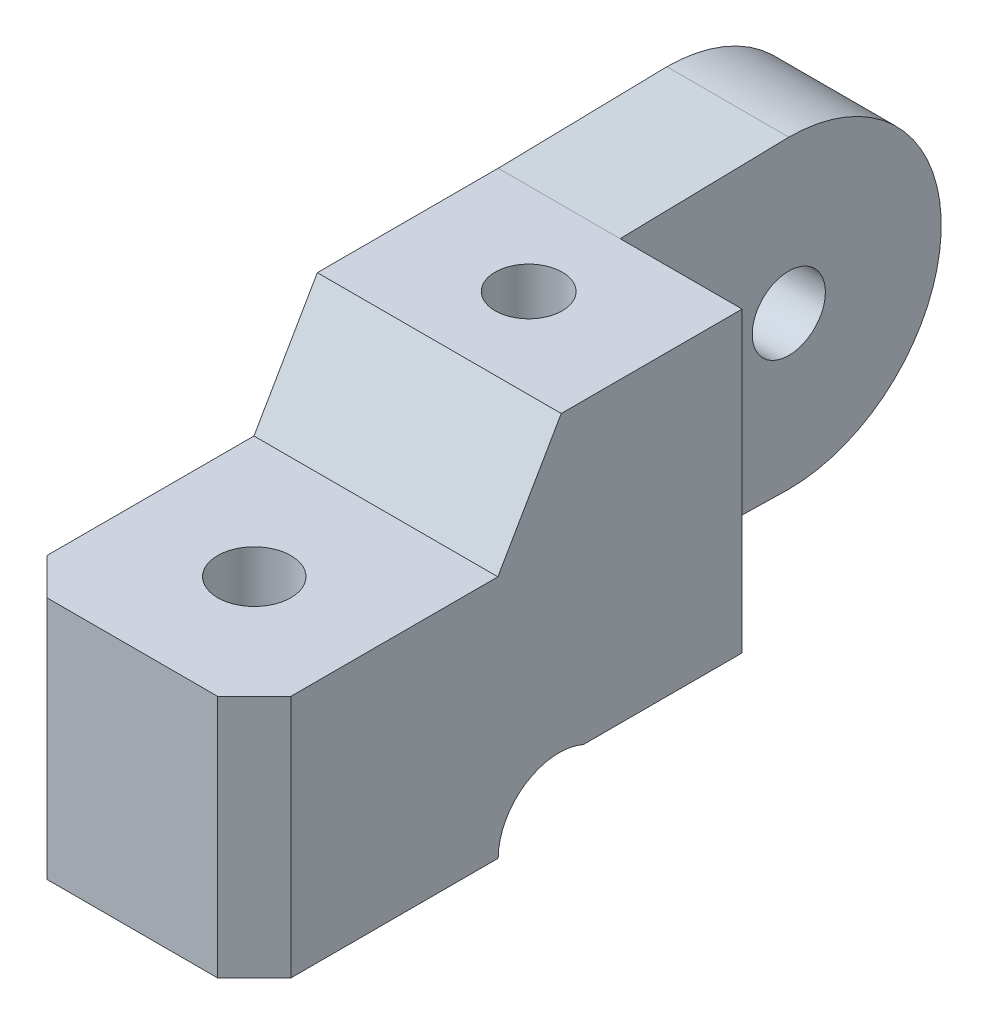
ISO-10303-21;
HEADER;
FILE_DESCRIPTION(('STEP AP214'),'2;1');
FILE_NAME('part.step','',(''),(''),'','','');
FILE_SCHEMA(('AUTOMOTIVE_DESIGN { 1 0 10303 214 1 1 1 1 }'));
ENDSEC;
DATA;
#1=APPLICATION_CONTEXT('core data for automotive mechanical design processes');
#2=APPLICATION_PROTOCOL_DEFINITION('international standard','automotive_design',2000,#1);
#3=PRODUCT_CONTEXT('',#1,'mechanical');
#4=PRODUCT('Part','Part','',(#3));
#5=PRODUCT_RELATED_PRODUCT_CATEGORY('part','',(#4));
#6=PRODUCT_DEFINITION_FORMATION('','',#4);
#7=PRODUCT_DEFINITION_CONTEXT('part definition',#1,'design');
#8=PRODUCT_DEFINITION('design','',#6,#7);
#9=PRODUCT_DEFINITION_SHAPE('','',#8);
#10=(LENGTH_UNIT() NAMED_UNIT(*) SI_UNIT(.MILLI.,.METRE.));
#11=(NAMED_UNIT(*) PLANE_ANGLE_UNIT() SI_UNIT($,.RADIAN.));
#12=(NAMED_UNIT(*) SI_UNIT($,.STERADIAN.) SOLID_ANGLE_UNIT());
#13=UNCERTAINTY_MEASURE_WITH_UNIT(LENGTH_MEASURE(1.E-05),#10,'distance_accuracy_value','');
#14=(GEOMETRIC_REPRESENTATION_CONTEXT(3) GLOBAL_UNCERTAINTY_ASSIGNED_CONTEXT((#13)) GLOBAL_UNIT_ASSIGNED_CONTEXT((#10,
#11,#12)) REPRESENTATION_CONTEXT('',''));
#15=CARTESIAN_POINT('',(0.,0.,0.));
#16=DIRECTION('',(0.,0.,1.));
#17=DIRECTION('',(1.,0.,0.));
#18=AXIS2_PLACEMENT_3D('',#15,#16,#17);
#19=CARTESIAN_POINT('',(20.,9.16515138991168,-80.));
#20=DIRECTION('',(0.,0.,1.));
#21=DIRECTION('',(1.,0.,0.));
#22=AXIS2_PLACEMENT_3D('',#19,#20,#21);
#23=PLANE('',#22);
#24=DIRECTION('',(0.,-1.,0.));
#25=VECTOR('',#24,1.);
#26=CARTESIAN_POINT('',(0.,58.,-80.));
#27=LINE('',#26,#25);
#28=CARTESIAN_POINT('',(0.,58.,-80.));
#29=VERTEX_POINT('',#28);
#30=CARTESIAN_POINT('',(0.,9.16515138991168,-80.));
#31=VERTEX_POINT('',#30);
#32=EDGE_CURVE('E57',#29,#31,#27,.T.);
#33=ORIENTED_EDGE('',*,*,#32,.F.);
#34=DIRECTION('',(-1.,0.,0.));
#35=VECTOR('',#34,1.);
#36=CARTESIAN_POINT('',(20.,58.,-80.));
#37=LINE('',#36,#35);
#38=CARTESIAN_POINT('',(20.,58.,-80.));
#39=VERTEX_POINT('',#38);
#40=EDGE_CURVE('E142',#39,#29,#37,.T.);
#41=ORIENTED_EDGE('',*,*,#40,.F.);
#42=DIRECTION('',(0.,1.,0.));
#43=VECTOR('',#42,1.);
#44=CARTESIAN_POINT('',(20.,9.16515138991168,-80.));
#45=LINE('',#44,#43);
#46=CARTESIAN_POINT('',(20.,9.16515138991168,-80.));
#47=VERTEX_POINT('',#46);
#48=EDGE_CURVE('E140',#47,#39,#45,.T.);
#49=ORIENTED_EDGE('',*,*,#48,.F.);
#50=DIRECTION('',(-1.,0.,0.));
#51=VECTOR('',#50,1.);
#52=CARTESIAN_POINT('',(20.,9.16515138991168,-80.));
#53=LINE('',#52,#51);
#54=EDGE_CURVE('E132',#47,#31,#53,.T.);
#55=ORIENTED_EDGE('',*,*,#54,.T.);
#56=EDGE_LOOP('',(#33,#41,#49,#55));
#57=FACE_BOUND('',#56,.T.);
#58=ADVANCED_FACE('F41',(#57),#23,.F.);
#59=CARTESIAN_POINT('',(20.,40.,0.));
#60=DIRECTION('',(0.,0.,-1.));
#61=DIRECTION('',(0.,1.,0.));
#62=AXIS2_PLACEMENT_3D('',#59,#60,#61);
#63=PLANE('',#62);
#64=DIRECTION('',(-1.,0.,0.));
#65=VECTOR('',#64,1.);
#66=CARTESIAN_POINT('',(20.,40.,0.));
#67=LINE('',#66,#65);
#68=CARTESIAN_POINT('',(14.,40.,0.));
#69=VERTEX_POINT('',#68);
#70=CARTESIAN_POINT('',(-14.,40.,0.));
#71=VERTEX_POINT('',#70);
#72=EDGE_CURVE('E227',#69,#71,#67,.T.);
#73=ORIENTED_EDGE('',*,*,#72,.T.);
#74=DIRECTION('',(0.,-1.,0.));
#75=VECTOR('',#74,1.);
#76=CARTESIAN_POINT('',(-14.,58.,0.));
#77=LINE('',#76,#75);
#78=CARTESIAN_POINT('',(-14.,0.,0.));
#79=VERTEX_POINT('',#78);
#80=EDGE_CURVE('E197',#71,#79,#77,.T.);
#81=ORIENTED_EDGE('',*,*,#80,.T.);
#82=DIRECTION('',(-1.,0.,0.));
#83=VECTOR('',#82,1.);
#84=CARTESIAN_POINT('',(20.,0.,0.));
#85=LINE('',#84,#83);
#86=CARTESIAN_POINT('',(14.,0.,0.));
#87=VERTEX_POINT('',#86);
#88=EDGE_CURVE('E252',#87,#79,#85,.T.);
#89=ORIENTED_EDGE('',*,*,#88,.F.);
#90=DIRECTION('',(0.,-1.,0.));
#91=VECTOR('',#90,1.);
#92=CARTESIAN_POINT('',(14.,58.,0.));
#93=LINE('',#92,#91);
#94=EDGE_CURVE('E207',#69,#87,#93,.T.);
#95=ORIENTED_EDGE('',*,*,#94,.F.);
#96=EDGE_LOOP('',(#73,#81,#89,#95));
#97=FACE_BOUND('',#96,.T.);
#98=ADVANCED_FACE('F43',(#97),#63,.F.);
#99=CARTESIAN_POINT('',(20.,0.,0.));
#100=DIRECTION('',(0.,1.,0.));
#101=DIRECTION('',(0.,0.,1.));
#102=AXIS2_PLACEMENT_3D('',#99,#100,#101);
#103=PLANE('',#102);
#104=ORIENTED_EDGE('',*,*,#88,.T.);
#105=DIRECTION('',(0.707106781186548,0.,0.707106781186548));
#106=VECTOR('',#105,1.);
#107=CARTESIAN_POINT('',(-20.,0.,-6.));
#108=LINE('',#107,#106);
#109=CARTESIAN_POINT('',(-20.,0.,-6.));
#110=VERTEX_POINT('',#109);
#111=EDGE_CURVE('E198',#110,#79,#108,.T.);
#112=ORIENTED_EDGE('',*,*,#111,.F.);
#113=DIRECTION('',(0.,0.,-1.));
#114=VECTOR('',#113,1.);
#115=CARTESIAN_POINT('',(-20.,0.,0.));
#116=LINE('',#115,#114);
#117=CARTESIAN_POINT('',(-20.,0.,-40.));
#118=VERTEX_POINT('',#117);
#119=EDGE_CURVE('E212',#110,#118,#116,.T.);
#120=ORIENTED_EDGE('',*,*,#119,.T.);
#121=DIRECTION('',(-1.,0.,0.));
#122=VECTOR('',#121,1.);
#123=CARTESIAN_POINT('',(20.,0.,-40.));
#124=LINE('',#123,#122);
#125=CARTESIAN_POINT('',(20.,0.,-40.));
#126=VERTEX_POINT('',#125);
#127=EDGE_CURVE('E247',#126,#118,#124,.T.);
#128=ORIENTED_EDGE('',*,*,#127,.F.);
#129=DIRECTION('',(0.,0.,-1.));
#130=VECTOR('',#129,1.);
#131=CARTESIAN_POINT('',(20.,0.,0.));
#132=LINE('',#131,#130);
#133=CARTESIAN_POINT('',(20.,0.,-6.));
#134=VERTEX_POINT('',#133);
#135=EDGE_CURVE('E215',#134,#126,#132,.T.);
#136=ORIENTED_EDGE('',*,*,#135,.F.);
#137=DIRECTION('',(0.707106781186548,0.,-0.707106781186548));
#138=VECTOR('',#137,1.);
#139=CARTESIAN_POINT('',(14.,0.,0.));
#140=LINE('',#139,#138);
#141=EDGE_CURVE('E202',#87,#134,#140,.T.);
#142=ORIENTED_EDGE('',*,*,#141,.F.);
#143=EDGE_LOOP('',(#104,#112,#120,#128,#136,#142));
#144=FACE_BOUND('',#143,.T.);
#145=ADVANCED_FACE('F265',(#144),#103,.F.);
#146=CARTESIAN_POINT('',(20.,0.,-50.));
#147=DIRECTION('',(-1.,0.,0.));
#148=DIRECTION('',(0.,0.,1.));
#149=AXIS2_PLACEMENT_3D('',#146,#147,#148);
#150=CYLINDRICAL_SURFACE('',#149,10.);
#151=CARTESIAN_POINT('',(-20.,0.,-50.));
#152=DIRECTION('',(-1.,0.,0.));
#153=DIRECTION('',(0.,0.,1.));
#154=AXIS2_PLACEMENT_3D('',#151,#152,#153);
#155=CIRCLE('',#154,10.);
#156=CARTESIAN_POINT('',(-20.,9.16515138991168,-54.));
#157=VERTEX_POINT('',#156);
#158=EDGE_CURVE('E230',#118,#157,#155,.T.);
#159=ORIENTED_EDGE('',*,*,#158,.T.);
#160=DIRECTION('',(-1.,0.,0.));
#161=VECTOR('',#160,1.);
#162=CARTESIAN_POINT('',(20.,9.16515138991168,-54.));
#163=LINE('',#162,#161);
#164=CARTESIAN_POINT('',(20.,9.16515138991168,-54.));
#165=VERTEX_POINT('',#164);
#166=EDGE_CURVE('E139',#165,#157,#163,.T.);
#167=ORIENTED_EDGE('',*,*,#166,.F.);
#168=CARTESIAN_POINT('',(20.,0.,-50.));
#169=DIRECTION('',(-1.,0.,0.));
#170=DIRECTION('',(0.,0.,1.));
#171=AXIS2_PLACEMENT_3D('',#168,#169,#170);
#172=CIRCLE('',#171,10.);
#173=EDGE_CURVE('E211',#126,#165,#172,.T.);
#174=ORIENTED_EDGE('',*,*,#173,.F.);
#175=ORIENTED_EDGE('',*,*,#127,.T.);
#176=EDGE_LOOP('',(#159,#167,#174,#175));
#177=FACE_BOUND('',#176,.T.);
#178=ADVANCED_FACE('F269',(#177),#150,.F.);
#179=CARTESIAN_POINT('',(20.,9.16515138991168,-54.));
#180=DIRECTION('',(0.,1.,0.));
#181=DIRECTION('',(0.,0.,1.));
#182=AXIS2_PLACEMENT_3D('',#179,#180,#181);
#183=PLANE('',#182);
#184=DIRECTION('',(0.,0.,-1.));
#185=VECTOR('',#184,1.);
#186=CARTESIAN_POINT('',(-20.,9.16515138991168,-54.));
#187=LINE('',#186,#185);
#188=CARTESIAN_POINT('',(-20.,9.16515138991168,-80.));
#189=VERTEX_POINT('',#188);
#190=EDGE_CURVE('E149',#157,#189,#187,.T.);
#191=ORIENTED_EDGE('',*,*,#190,.T.);
#192=DIRECTION('',(-1.,0.,0.));
#193=VECTOR('',#192,1.);
#194=CARTESIAN_POINT('',(0.,9.16515138991168,-80.));
#195=LINE('',#194,#193);
#196=EDGE_CURVE('E144',#31,#189,#195,.T.);
#197=ORIENTED_EDGE('',*,*,#196,.F.);
#198=ORIENTED_EDGE('',*,*,#54,.F.);
#199=DIRECTION('',(0.,0.,-1.));
#200=VECTOR('',#199,1.);
#201=CARTESIAN_POINT('',(20.,9.16515138991168,-54.));
#202=LINE('',#201,#200);
#203=EDGE_CURVE('E220',#165,#47,#202,.T.);
#204=ORIENTED_EDGE('',*,*,#203,.F.);
#205=ORIENTED_EDGE('',*,*,#166,.T.);
#206=EDGE_LOOP('',(#191,#197,#198,#204,#205));
#207=FACE_BOUND('',#206,.T.);
#208=ADVANCED_FACE('F143',(#207),#183,.F.);
#209=CARTESIAN_POINT('',(20.,58.,-80.));
#210=DIRECTION('',(0.,-1.,0.));
#211=DIRECTION('',(0.,0.,-1.));
#212=AXIS2_PLACEMENT_3D('',#209,#210,#211);
#213=PLANE('',#212);
#214=CARTESIAN_POINT('',(0.,58.,-65.));
#215=DIRECTION('',(0.,1.,0.));
#216=DIRECTION('',(0.,0.,1.));
#217=AXIS2_PLACEMENT_3D('',#214,#215,#216);
#218=CIRCLE('',#217,5.5);
#219=CARTESIAN_POINT('',(0.,58.,-59.5));
#220=VERTEX_POINT('',#219);
#221=EDGE_CURVE('E187',#220,#220,#218,.T.);
#222=ORIENTED_EDGE('',*,*,#221,.F.);
#223=EDGE_LOOP('',(#222));
#224=FACE_BOUND('',#223,.T.);
#225=DIRECTION('',(0.,0.,1.));
#226=VECTOR('',#225,1.);
#227=CARTESIAN_POINT('',(-20.,58.,-80.));
#228=LINE('',#227,#226);
#229=CARTESIAN_POINT('',(-20.,58.,-80.));
#230=VERTEX_POINT('',#229);
#231=CARTESIAN_POINT('',(-20.,58.,-50.3413947328154));
#232=VERTEX_POINT('',#231);
#233=EDGE_CURVE('E235',#230,#232,#228,.T.);
#234=ORIENTED_EDGE('',*,*,#233,.T.);
#235=DIRECTION('',(-1.,0.,0.));
#236=VECTOR('',#235,1.);
#237=CARTESIAN_POINT('',(20.,58.,-50.3413947328154));
#238=LINE('',#237,#236);
#239=CARTESIAN_POINT('',(20.,58.,-50.3413947328154));
#240=VERTEX_POINT('',#239);
#241=EDGE_CURVE('E243',#240,#232,#238,.T.);
#242=ORIENTED_EDGE('',*,*,#241,.F.);
#243=DIRECTION('',(0.,0.,1.));
#244=VECTOR('',#243,1.);
#245=CARTESIAN_POINT('',(20.,58.,-80.));
#246=LINE('',#245,#244);
#247=EDGE_CURVE('E217',#39,#240,#246,.T.);
#248=ORIENTED_EDGE('',*,*,#247,.F.);
#249=ORIENTED_EDGE('',*,*,#40,.T.);
#250=DIRECTION('',(-1.,0.,0.));
#251=VECTOR('',#250,1.);
#252=CARTESIAN_POINT('',(0.,58.,-80.));
#253=LINE('',#252,#251);
#254=EDGE_CURVE('E151',#29,#230,#253,.T.);
#255=ORIENTED_EDGE('',*,*,#254,.T.);
#256=EDGE_LOOP('',(#234,#242,#248,#249,#255));
#257=FACE_BOUND('',#256,.T.);
#258=ADVANCED_FACE('F311',(#224,#257),#213,.F.);
#259=CARTESIAN_POINT('',(20.,58.,-50.3413947328154));
#260=DIRECTION('',(0.,-0.499999999999998,-0.86602540378444));
#261=DIRECTION('',(0.,0.86602540378444,-0.499999999999998));
#262=AXIS2_PLACEMENT_3D('',#259,#260,#261);
#263=PLANE('',#262);
#264=DIRECTION('',(0.,-0.86602540378444,0.499999999999998));
#265=VECTOR('',#264,1.);
#266=CARTESIAN_POINT('',(-20.,58.,-50.3413947328154));
#267=LINE('',#266,#265);
#268=CARTESIAN_POINT('',(-20.,40.,-39.9490898874022));
#269=VERTEX_POINT('',#268);
#270=EDGE_CURVE('E234',#232,#269,#267,.T.);
#271=ORIENTED_EDGE('',*,*,#270,.T.);
#272=DIRECTION('',(-1.,0.,0.));
#273=VECTOR('',#272,1.);
#274=CARTESIAN_POINT('',(20.,40.,-39.9490898874022));
#275=LINE('',#274,#273);
#276=CARTESIAN_POINT('',(20.,40.,-39.9490898874022));
#277=VERTEX_POINT('',#276);
#278=EDGE_CURVE('E239',#277,#269,#275,.T.);
#279=ORIENTED_EDGE('',*,*,#278,.F.);
#280=DIRECTION('',(0.,-0.86602540378444,0.499999999999998));
#281=VECTOR('',#280,1.);
#282=CARTESIAN_POINT('',(20.,58.,-50.3413947328154));
#283=LINE('',#282,#281);
#284=EDGE_CURVE('E225',#240,#277,#283,.T.);
#285=ORIENTED_EDGE('',*,*,#284,.F.);
#286=ORIENTED_EDGE('',*,*,#241,.T.);
#287=EDGE_LOOP('',(#271,#279,#285,#286));
#288=FACE_BOUND('',#287,.T.);
#289=ADVANCED_FACE('F345',(#288),#263,.F.);
#290=CARTESIAN_POINT('',(20.,40.,-39.9490898874022));
#291=DIRECTION('',(0.,-1.,0.));
#292=DIRECTION('',(0.,0.,-1.));
#293=AXIS2_PLACEMENT_3D('',#290,#291,#292);
#294=PLANE('',#293);
#295=CARTESIAN_POINT('',(0.,40.,-20.));
#296=DIRECTION('',(0.,1.,0.));
#297=DIRECTION('',(0.,0.,1.));
#298=AXIS2_PLACEMENT_3D('',#295,#296,#297);
#299=CIRCLE('',#298,6.);
#300=CARTESIAN_POINT('',(0.,40.,-14.));
#301=VERTEX_POINT('',#300);
#302=EDGE_CURVE('E188',#301,#301,#299,.T.);
#303=ORIENTED_EDGE('',*,*,#302,.F.);
#304=EDGE_LOOP('',(#303));
#305=FACE_BOUND('',#304,.T.);
#306=DIRECTION('',(0.,0.,1.));
#307=VECTOR('',#306,1.);
#308=CARTESIAN_POINT('',(-20.,40.,-39.9490898874022));
#309=LINE('',#308,#307);
#310=CARTESIAN_POINT('',(-20.,40.,-6.));
#311=VERTEX_POINT('',#310);
#312=EDGE_CURVE('E213',#269,#311,#309,.T.);
#313=ORIENTED_EDGE('',*,*,#312,.T.);
#314=DIRECTION('',(0.707106781186548,0.,0.707106781186548));
#315=VECTOR('',#314,1.);
#316=CARTESIAN_POINT('',(-16.9745449437011,40.,-2.97454494370112));
#317=LINE('',#316,#315);
#318=EDGE_CURVE('E64',#311,#71,#317,.T.);
#319=ORIENTED_EDGE('',*,*,#318,.T.);
#320=ORIENTED_EDGE('',*,*,#72,.F.);
#321=DIRECTION('',(0.707106781186548,0.,-0.707106781186548));
#322=VECTOR('',#321,1.);
#323=CARTESIAN_POINT('',(36.9745449437011,40.,-22.9745449437011));
#324=LINE('',#323,#322);
#325=CARTESIAN_POINT('',(20.,40.,-6.));
#326=VERTEX_POINT('',#325);
#327=EDGE_CURVE('E206',#69,#326,#324,.T.);
#328=ORIENTED_EDGE('',*,*,#327,.T.);
#329=DIRECTION('',(0.,0.,1.));
#330=VECTOR('',#329,1.);
#331=CARTESIAN_POINT('',(20.,40.,-39.9490898874022));
#332=LINE('',#331,#330);
#333=EDGE_CURVE('E222',#277,#326,#332,.T.);
#334=ORIENTED_EDGE('',*,*,#333,.F.);
#335=ORIENTED_EDGE('',*,*,#278,.T.);
#336=EDGE_LOOP('',(#313,#319,#320,#328,#334,#335));
#337=FACE_BOUND('',#336,.T.);
#338=ADVANCED_FACE('F336',(#305,#337),#294,.F.);
#339=CARTESIAN_POINT('',(20.,0.,-50.));
#340=DIRECTION('',(-1.,0.,0.));
#341=DIRECTION('',(0.,0.,1.));
#342=AXIS2_PLACEMENT_3D('',#339,#340,#341);
#343=PLANE('',#342);
#344=ORIENTED_EDGE('',*,*,#333,.T.);
#345=DIRECTION('',(0.,-1.,0.));
#346=VECTOR('',#345,1.);
#347=CARTESIAN_POINT('',(20.,0.,-5.99999999999999));
#348=LINE('',#347,#346);
#349=EDGE_CURVE('E47',#326,#134,#348,.T.);
#350=ORIENTED_EDGE('',*,*,#349,.T.);
#351=ORIENTED_EDGE('',*,*,#135,.T.);
#352=ORIENTED_EDGE('',*,*,#173,.T.);
#353=ORIENTED_EDGE('',*,*,#203,.T.);
#354=ORIENTED_EDGE('',*,*,#48,.T.);
#355=ORIENTED_EDGE('',*,*,#247,.T.);
#356=ORIENTED_EDGE('',*,*,#284,.T.);
#357=EDGE_LOOP('',(#344,#350,#351,#352,#353,#354,#355,#356));
#358=FACE_BOUND('',#357,.T.);
#359=ADVANCED_FACE('F257',(#358),#343,.F.);
#360=CARTESIAN_POINT('',(-20.,0.,-50.));
#361=DIRECTION('',(-1.,0.,0.));
#362=DIRECTION('',(0.,0.,1.));
#363=AXIS2_PLACEMENT_3D('',#360,#361,#362);
#364=PLANE('',#363);
#365=CARTESIAN_POINT('',(-20.,33.5825756949558,-107.657336828865));
#366=DIRECTION('',(1.,0.,0.));
#367=DIRECTION('',(0.,0.,-1.));
#368=AXIS2_PLACEMENT_3D('',#365,#366,#367);
#369=CIRCLE('',#368,6.);
#370=CARTESIAN_POINT('',(-20.,33.5825756949558,-113.657336828865));
#371=VERTEX_POINT('',#370);
#372=EDGE_CURVE('E178',#371,#371,#369,.T.);
#373=ORIENTED_EDGE('',*,*,#372,.T.);
#374=EDGE_LOOP('',(#373));
#375=FACE_BOUND('',#374,.T.);
#376=DIRECTION('',(0.,-1.,0.));
#377=VECTOR('',#376,1.);
#378=CARTESIAN_POINT('',(-20.,0.,-6.));
#379=LINE('',#378,#377);
#380=EDGE_CURVE('E11',#311,#110,#379,.T.);
#381=ORIENTED_EDGE('',*,*,#380,.F.);
#382=ORIENTED_EDGE('',*,*,#312,.F.);
#383=ORIENTED_EDGE('',*,*,#270,.F.);
#384=ORIENTED_EDGE('',*,*,#233,.F.);
#385=DIRECTION('',(0.,-0.0210593846670048,0.999778226566996));
#386=VECTOR('',#385,1.);
#387=CARTESIAN_POINT('',(-20.,58.5825756949559,-107.657336828865));
#388=LINE('',#387,#386);
#389=CARTESIAN_POINT('',(-20.,58.5825756949559,-107.657336828865));
#390=VERTEX_POINT('',#389);
#391=EDGE_CURVE('E172',#390,#230,#388,.T.);
#392=ORIENTED_EDGE('',*,*,#391,.F.);
#393=CARTESIAN_POINT('',(-20.,33.5825756949558,-107.657336828865));
#394=DIRECTION('',(-1.,0.,0.));
#395=DIRECTION('',(0.,0.,1.));
#396=AXIS2_PLACEMENT_3D('',#393,#394,#395);
#397=CIRCLE('',#396,25.);
#398=CARTESIAN_POINT('',(-20.,8.58257569495584,-107.657336828865));
#399=VERTEX_POINT('',#398);
#400=EDGE_CURVE('E179',#390,#399,#397,.T.);
#401=ORIENTED_EDGE('',*,*,#400,.T.);
#402=DIRECTION('',(0.,-0.0210593846670045,-0.999778226566996));
#403=VECTOR('',#402,1.);
#404=CARTESIAN_POINT('',(-20.,9.16515138991168,-80.));
#405=LINE('',#404,#403);
#406=EDGE_CURVE('E180',#189,#399,#405,.T.);
#407=ORIENTED_EDGE('',*,*,#406,.F.);
#408=ORIENTED_EDGE('',*,*,#190,.F.);
#409=ORIENTED_EDGE('',*,*,#158,.F.);
#410=ORIENTED_EDGE('',*,*,#119,.F.);
#411=EDGE_LOOP('',(#381,#382,#383,#384,#392,#401,#407,#408,#409,#410));
#412=FACE_BOUND('',#411,.T.);
#413=ADVANCED_FACE('F275',(#375,#412),#364,.T.);
#414=CARTESIAN_POINT('',(14.,58.,0.));
#415=DIRECTION('',(-0.707106781186548,0.,-0.707106781186548));
#416=DIRECTION('',(-0.707106781186548,0.,0.707106781186548));
#417=AXIS2_PLACEMENT_3D('',#414,#415,#416);
#418=PLANE('',#417);
#419=ORIENTED_EDGE('',*,*,#94,.T.);
#420=ORIENTED_EDGE('',*,*,#141,.T.);
#421=ORIENTED_EDGE('',*,*,#349,.F.);
#422=ORIENTED_EDGE('',*,*,#327,.F.);
#423=EDGE_LOOP('',(#419,#420,#421,#422));
#424=FACE_BOUND('',#423,.T.);
#425=ADVANCED_FACE('F333',(#424),#418,.F.);
#426=CARTESIAN_POINT('',(-20.,58.,-6.));
#427=DIRECTION('',(0.707106781186548,0.,-0.707106781186548));
#428=DIRECTION('',(-0.707106781186548,0.,-0.707106781186548));
#429=AXIS2_PLACEMENT_3D('',#426,#427,#428);
#430=PLANE('',#429);
#431=ORIENTED_EDGE('',*,*,#380,.T.);
#432=ORIENTED_EDGE('',*,*,#111,.T.);
#433=ORIENTED_EDGE('',*,*,#80,.F.);
#434=ORIENTED_EDGE('',*,*,#318,.F.);
#435=EDGE_LOOP('',(#431,#432,#433,#434));
#436=FACE_BOUND('',#435,.T.);
#437=ADVANCED_FACE('F328',(#436),#430,.F.);
#438=CARTESIAN_POINT('',(0.,29.,-20.));
#439=DIRECTION('',(0.,1.,0.));
#440=DIRECTION('',(0.,0.,1.));
#441=AXIS2_PLACEMENT_3D('',#438,#439,#440);
#442=CYLINDRICAL_SURFACE('',#441,6.);
#443=CARTESIAN_POINT('',(0.,29.,-20.));
#444=DIRECTION('',(0.,1.,0.));
#445=DIRECTION('',(0.,0.,1.));
#446=AXIS2_PLACEMENT_3D('',#443,#444,#445);
#447=CIRCLE('',#446,6.);
#448=CARTESIAN_POINT('',(0.,29.,-14.));
#449=VERTEX_POINT('',#448);
#450=EDGE_CURVE('E194',#449,#449,#447,.T.);
#451=ORIENTED_EDGE('',*,*,#450,.F.);
#452=EDGE_LOOP('',(#451));
#453=FACE_BOUND('',#452,.T.);
#454=ORIENTED_EDGE('',*,*,#302,.T.);
#455=EDGE_LOOP('',(#454));
#456=FACE_BOUND('',#455,.T.);
#457=ADVANCED_FACE('F327',(#453,#456),#442,.F.);
#458=CARTESIAN_POINT('',(0.,29.,-20.));
#459=DIRECTION('',(0.,1.,0.));
#460=DIRECTION('',(0.,0.,1.));
#461=AXIS2_PLACEMENT_3D('',#458,#459,#460);
#462=PLANE('',#461);
#463=ORIENTED_EDGE('',*,*,#450,.T.);
#464=EDGE_LOOP('',(#463));
#465=FACE_BOUND('',#464,.T.);
#466=ADVANCED_FACE('F355',(#465),#462,.T.);
#467=CARTESIAN_POINT('',(0.,47.,-65.));
#468=DIRECTION('',(0.,1.,0.));
#469=DIRECTION('',(0.,0.,1.));
#470=AXIS2_PLACEMENT_3D('',#467,#468,#469);
#471=CYLINDRICAL_SURFACE('',#470,5.5);
#472=CARTESIAN_POINT('',(0.,47.,-65.));
#473=DIRECTION('',(0.,1.,0.));
#474=DIRECTION('',(0.,0.,1.));
#475=AXIS2_PLACEMENT_3D('',#472,#473,#474);
#476=CIRCLE('',#475,5.5);
#477=CARTESIAN_POINT('',(0.,47.,-59.5));
#478=VERTEX_POINT('',#477);
#479=EDGE_CURVE('E190',#478,#478,#476,.T.);
#480=ORIENTED_EDGE('',*,*,#479,.F.);
#481=EDGE_LOOP('',(#480));
#482=FACE_BOUND('',#481,.T.);
#483=ORIENTED_EDGE('',*,*,#221,.T.);
#484=EDGE_LOOP('',(#483));
#485=FACE_BOUND('',#484,.T.);
#486=ADVANCED_FACE('F363',(#482,#485),#471,.F.);
#487=CARTESIAN_POINT('',(0.,47.,-65.));
#488=DIRECTION('',(0.,1.,0.));
#489=DIRECTION('',(0.,0.,1.));
#490=AXIS2_PLACEMENT_3D('',#487,#488,#489);
#491=PLANE('',#490);
#492=ORIENTED_EDGE('',*,*,#479,.T.);
#493=EDGE_LOOP('',(#492));
#494=FACE_BOUND('',#493,.T.);
#495=ADVANCED_FACE('F367',(#494),#491,.T.);
#496=CARTESIAN_POINT('',(0.,58.5825756949559,-107.657336828865));
#497=DIRECTION('',(0.,-0.999778226566996,-0.0210593846670048));
#498=DIRECTION('',(0.,0.0210593846670048,-0.999778226566996));
#499=AXIS2_PLACEMENT_3D('',#496,#497,#498);
#500=PLANE('',#499);
#501=ORIENTED_EDGE('',*,*,#391,.T.);
#502=ORIENTED_EDGE('',*,*,#254,.F.);
#503=DIRECTION('',(0.,-0.0210593846670048,0.999778226566996));
#504=VECTOR('',#503,1.);
#505=CARTESIAN_POINT('',(0.,58.5825756949559,-107.657336828865));
#506=LINE('',#505,#504);
#507=CARTESIAN_POINT('',(0.,58.5825756949559,-107.657336828865));
#508=VERTEX_POINT('',#507);
#509=EDGE_CURVE('E161',#508,#29,#506,.T.);
#510=ORIENTED_EDGE('',*,*,#509,.F.);
#511=DIRECTION('',(-1.,0.,0.));
#512=VECTOR('',#511,1.);
#513=CARTESIAN_POINT('',(0.,58.5825756949559,-107.657336828865));
#514=LINE('',#513,#512);
#515=EDGE_CURVE('E167',#508,#390,#514,.T.);
#516=ORIENTED_EDGE('',*,*,#515,.T.);
#517=EDGE_LOOP('',(#501,#502,#510,#516));
#518=FACE_BOUND('',#517,.T.);
#519=ADVANCED_FACE('F276',(#518),#500,.F.);
#520=CARTESIAN_POINT('',(0.,9.16515138991168,-80.));
#521=DIRECTION('',(0.,0.999778226566996,-0.0210593846670045));
#522=DIRECTION('',(0.,0.0210593846670045,0.999778226566996));
#523=AXIS2_PLACEMENT_3D('',#520,#521,#522);
#524=PLANE('',#523);
#525=ORIENTED_EDGE('',*,*,#406,.T.);
#526=DIRECTION('',(-1.,0.,0.));
#527=VECTOR('',#526,1.);
#528=CARTESIAN_POINT('',(0.,8.58257569495584,-107.657336828865));
#529=LINE('',#528,#527);
#530=CARTESIAN_POINT('',(0.,8.58257569495584,-107.657336828865));
#531=VERTEX_POINT('',#530);
#532=EDGE_CURVE('E154',#531,#399,#529,.T.);
#533=ORIENTED_EDGE('',*,*,#532,.F.);
#534=DIRECTION('',(0.,-0.0210593846670045,-0.999778226566996));
#535=VECTOR('',#534,1.);
#536=CARTESIAN_POINT('',(0.,9.16515138991168,-80.));
#537=LINE('',#536,#535);
#538=EDGE_CURVE('E159',#31,#531,#537,.T.);
#539=ORIENTED_EDGE('',*,*,#538,.F.);
#540=ORIENTED_EDGE('',*,*,#196,.T.);
#541=EDGE_LOOP('',(#525,#533,#539,#540));
#542=FACE_BOUND('',#541,.T.);
#543=ADVANCED_FACE('F168',(#542),#524,.F.);
#544=CARTESIAN_POINT('',(0.,33.5825756949558,-107.657336828865));
#545=DIRECTION('',(-1.,0.,0.));
#546=DIRECTION('',(0.,0.,1.));
#547=AXIS2_PLACEMENT_3D('',#544,#545,#546);
#548=CYLINDRICAL_SURFACE('',#547,25.);
#549=ORIENTED_EDGE('',*,*,#400,.F.);
#550=ORIENTED_EDGE('',*,*,#515,.F.);
#551=CARTESIAN_POINT('',(0.,33.5825756949558,-107.657336828865));
#552=DIRECTION('',(-1.,0.,0.));
#553=DIRECTION('',(0.,0.,1.));
#554=AXIS2_PLACEMENT_3D('',#551,#552,#553);
#555=CIRCLE('',#554,25.);
#556=EDGE_CURVE('E166',#508,#531,#555,.T.);
#557=ORIENTED_EDGE('',*,*,#556,.T.);
#558=ORIENTED_EDGE('',*,*,#532,.T.);
#559=EDGE_LOOP('',(#549,#550,#557,#558));
#560=FACE_BOUND('',#559,.T.);
#561=ADVANCED_FACE('F280',(#560),#548,.T.);
#562=CARTESIAN_POINT('',(0.,33.5825756949558,-107.657336828865));
#563=DIRECTION('',(-1.,0.,0.));
#564=DIRECTION('',(0.,0.,1.));
#565=AXIS2_PLACEMENT_3D('',#562,#563,#564);
#566=PLANE('',#565);
#567=CARTESIAN_POINT('',(0.,33.5825756949558,-107.657336828865));
#568=DIRECTION('',(1.,0.,0.));
#569=DIRECTION('',(0.,0.,-1.));
#570=AXIS2_PLACEMENT_3D('',#567,#568,#569);
#571=CIRCLE('',#570,6.);
#572=CARTESIAN_POINT('',(0.,33.5825756949558,-113.657336828865));
#573=VERTEX_POINT('',#572);
#574=EDGE_CURVE('E283',#573,#573,#571,.T.);
#575=ORIENTED_EDGE('',*,*,#574,.F.);
#576=EDGE_LOOP('',(#575));
#577=FACE_BOUND('',#576,.T.);
#578=ORIENTED_EDGE('',*,*,#509,.T.);
#579=ORIENTED_EDGE('',*,*,#32,.T.);
#580=ORIENTED_EDGE('',*,*,#538,.T.);
#581=ORIENTED_EDGE('',*,*,#556,.F.);
#582=EDGE_LOOP('',(#578,#579,#580,#581));
#583=FACE_BOUND('',#582,.T.);
#584=ADVANCED_FACE('F156',(#577,#583),#566,.F.);
#585=CARTESIAN_POINT('',(-20.,33.5825756949558,-107.657336828865));
#586=DIRECTION('',(1.,0.,0.));
#587=DIRECTION('',(0.,0.,-1.));
#588=AXIS2_PLACEMENT_3D('',#585,#586,#587);
#589=CYLINDRICAL_SURFACE('',#588,6.);
#590=ORIENTED_EDGE('',*,*,#372,.F.);
#591=EDGE_LOOP('',(#590));
#592=FACE_BOUND('',#591,.T.);
#593=ORIENTED_EDGE('',*,*,#574,.T.);
#594=EDGE_LOOP('',(#593));
#595=FACE_BOUND('',#594,.T.);
#596=ADVANCED_FACE('F286',(#592,#595),#589,.F.);
#597=CLOSED_SHELL('',(#58,#98,#145,#178,#208,#258,#289,#338,#359,#413,#425,#437,#457,#466,#486,
#495,#519,#543,#561,#584,#596));
#598=MANIFOLD_SOLID_BREP('B2',#597);
#599=ADVANCED_BREP_SHAPE_REPRESENTATION('',(#18,#598),#14);
#600=SHAPE_DEFINITION_REPRESENTATION(#9,#599);
ENDSEC;
END-ISO-10303-21;
